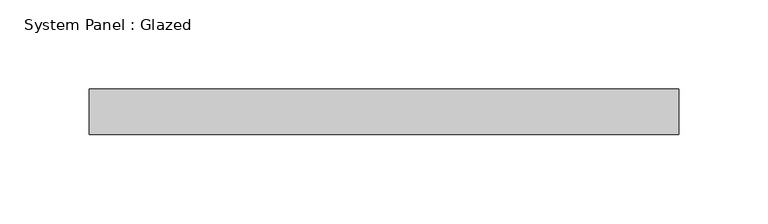
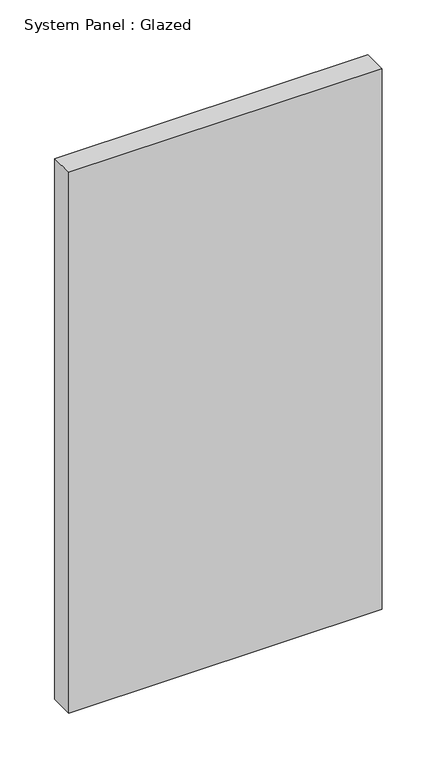
"""IFC4 building model written with IfcOpenShell, lengths in millimetres: plate geometry, System Panel : Glazed."""

from ifc_helpers import new_model, si_unit, origin, origin_with_axes, place, context, project, spatial, polyline, outline, extrude, source, transform, mapped, element, save


def system_panel_glazed_d4755e25(model_context):
    return source(origin(), model_context, "Body", "SweptSolid", [
        extrude(outline(polyline([(165.1, 19.05), (-165.1, 19.05), (-165.1, 44.45), (165.1, 44.45), (165.1, 19.05)])), origin_with_axes(), (0.0, 0.0, 1.0), 602.0842307),
    ])


if __name__ == "__main__":
    model = new_model("IFC4")
    model_context = context("Model", 3, world=origin())
    ifc_project = project(units=[si_unit("LENGTHUNIT", "METRE", prefix="MILLI")], contexts=[model_context])
    site = spatial("IfcSite", under=ifc_project)
    building = spatial("IfcBuilding", under=site)
    placement = place(None, origin())
    system_panel_glazed_shape = system_panel_glazed_d4755e25(model_context)
    element("IfcPlate", 1, ObjectType="System Panel : Glazed", at=placement, inside=building, context=model_context, shape_type="MappedRepresentation", body=[
        mapped(system_panel_glazed_shape, transform((0.0, 0.0, 0.0), x_axis=(1.0, 0.0, 0.0), y_axis=(0.0, 1.0, 0.0), z_axis=(0.0, 0.0, 1.0))),
    ])
    save(model, "model.ifc")

# Revit data of these elements
# Type "System Panel : Glazed"
#   Construction Type Id = "GSP4R"
#   Analytic Construction = "1/8 in Pilkington single glazing"
#   Visual Light Transmittance = 0.9
#   Solar Heat Gain Coefficient = 0.86
#   Heat Transfer Coefficient (U) = 1.18115 BTU/(h·ft²·°F)
#   Define Thermal Properties by = 1
# Element 1 (IfcPlate, "System Panel : Glazed")
#   Materials on its faces: "Glass"
# Materials
#   "Glass": class "Glass", colour RGB 0 128 192, transparency 0.75, Description = "Soda Lime Glass", Cost = 0
